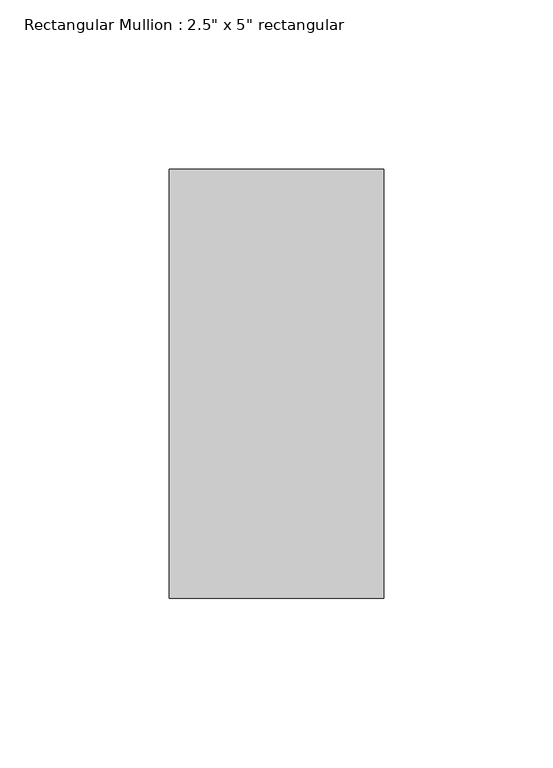
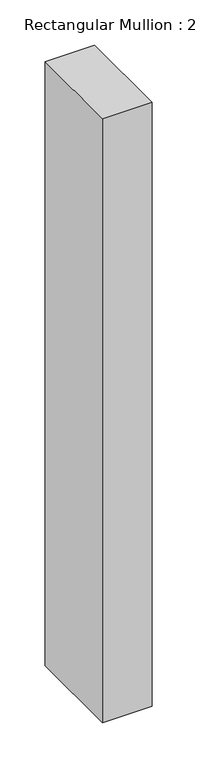
"""IFC4 building model written with IfcOpenShell, lengths in millimetres: member geometry."""

from ifc_helpers import new_model, si_unit, frame, origin, place, context, project, spatial, polyline, outline, extrude, source, transform, mapped, element, save


def member_8acf8d94(model_context):
    return source(origin(), model_context, "Body", "SweptSolid", [
        extrude(outline(polyline([(0.0, 63.5), (0.0, -63.5), (-63.5, -63.5), (-63.5, 63.5), (0.0, 63.5)])), frame((0.0, 0.0, -815.975), z_axis=(0.0, 0.0, 1.0), x_axis=(1.0, 0.0, 0.0)), (0.0, 0.0, 1.0), 815.975),
    ])


if __name__ == "__main__":
    model = new_model("IFC4")
    model_context = context("Model", 3, world=origin())
    ifc_project = project(units=[si_unit("LENGTHUNIT", "METRE", prefix="MILLI")], contexts=[model_context])
    site = spatial("IfcSite", under=ifc_project)
    building = spatial("IfcBuilding", under=site)
    placement = place(None, origin())
    member_shape = member_8acf8d94(model_context)
    element("IfcMember", 1, ObjectType="Rectangular Mullion : 2.5\" x 5\" rectangular", at=placement, inside=building, context=model_context, shape_type="MappedRepresentation", body=[
        mapped(member_shape, transform((0.0, 0.0, 0.0), x_axis=(1.0, 0.0, 0.0), y_axis=(0.0, 1.0, 0.0), z_axis=(0.0, 0.0, 1.0))),
    ])
    save(model, "model.ifc")

# Revit data of these elements
# Type "Rectangular Mullion : 2.5\" x 5\" rectangular"
#   built-in parameter 1007304 = 0.416667 (stored number, unit not read)
#   built-in parameter 1007301 = 0.104167 (stored number, unit not read)
#   built-in parameter 1007300 = 0.104167 (stored number, unit not read)
# Element 1 (IfcMember, "Rectangular Mullion : 2.5\" x 5\" rectangular")
#   Materials on its faces: "Aluminum"
# Materials
#   "Aluminum": class "Metal", colour RGB 247 247 247, transparency 0, Description = "Aluminum 6061", Cost = 0
